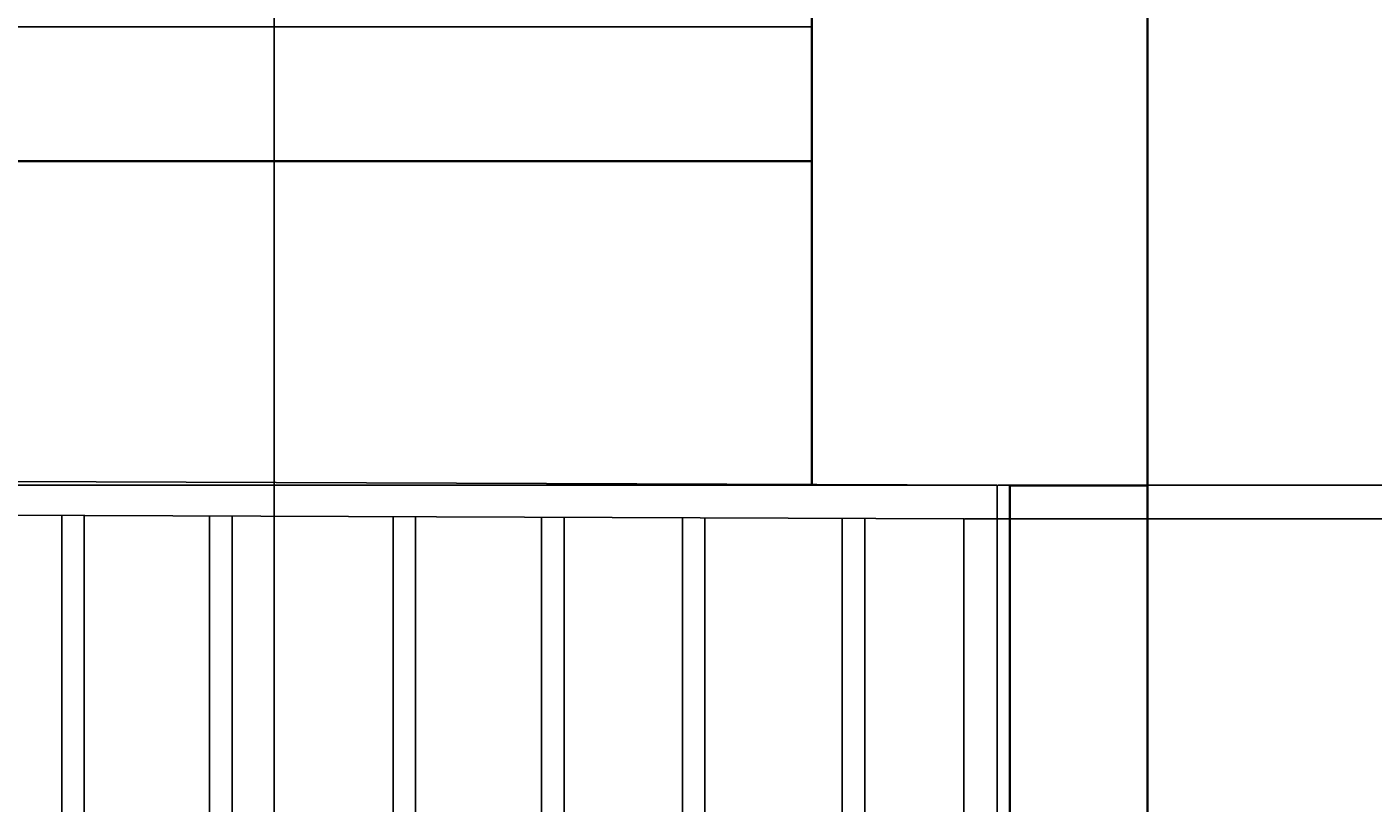
# Model space of a CAD drawing. Units: inches. Extents: x -13 to 809, y 112 to 656.
# Tile 42 of 55: x 521 to 641, y 181 to 251. Entities that reach past the tile are written whole.
import ezdxf

# ---------------------------------------------------------------- set-up
doc = ezdxf.new("R2010")
doc.units = ezdxf.units.IN
doc.header["$MEASUREMENT"] = 0
for name, color, linetype, lineweight in [('A-ANNO-DIMS', 2, 'Continuous', 18), ('A-DOOR', 4, 'Continuous', 25), ('A-ELEV', 7, 'Continuous', 35)]:
    doc.layers.add(name, color=color, linetype=linetype, lineweight=lineweight)
doc.styles.get("Standard").update_dxf_attribs({"font": 'arial.ttf'})
doc.dimstyles.get("Standard").update_dxf_attribs({"dimtxt": 0.625, "dimasz": 0.18, "dimexe": 0.18, "dimexo": 0.0625, "dimgap": 0.09, "dimtad": 0, "dimtih": 1, "dimtoh": 1, "dimdec": 4, "dimzin": 0, "dimdsep": 46, "dimlunit": 4, "dimtxsty": 'Standard', "dimcen": 0.09, "dimadec": 0, "dimazin": 0, "dimtfac": 1, "dimtdec": 4, "dimtofl": 0, "dimtmove": 0, "dimatfit": 3, "dimfxl": 1, "dimtolj": 1, "dimtzin": 0, "dimarcsym": 0})

# ---------------------------------------------------------------- blocks, each defined once
blk = doc.blocks.new('*D20')
at = {"layer": 'A-ANNO-DIMS', "color": 0, "lineweight": -2, "transparency": 16777216}
for p, q in [((365.94, 210.72), (365.94, 112.34)), ((607.57, 209.81), (607.57, 112.34)), ((366.12, 112.52), (485.36, 112.52)), ((607.39, 112.52), (488.15, 112.52))]:
    blk.add_line(p, q, dxfattribs=at)
at = {"layer": 'A-ANNO-DIMS', "color": 0, "transparency": 16777216}
for points in [[(366.12, 112.55), (366.12, 112.49), (365.94, 112.52)], [(607.39, 112.55), (607.39, 112.49), (607.57, 112.52)]]:
    blk.add_solid(points, dxfattribs=at)
at = {"layer": 'Defpoints', "color": 0, "transparency": 16777216}
for p in [(365.94, 210.78), (607.57, 209.88), (607.57, 112.52)]:
    blk.add_point(p, dxfattribs=at)
at = {"layer": 'A-ANNO-DIMS', "color": 0, "transparency": 16777216, "insert": (486.76, 112.52), "char_height": 0.625, "attachment_point": 5}
blk.add_mtext('\\A1;241.64', dxfattribs=at)
blk = doc.blocks.new('*D21')
at = {"layer": 'A-ANNO-DIMS', "color": 0, "lineweight": -2, "transparency": 16777216}
for p, q in [((607.57, 209.81), (607.57, 112.34)), ((621.01, 150.46), (621.01, 112.34)), ((607.75, 112.52), (612.93, 112.52)), ((620.83, 112.52), (615.65, 112.52))]:
    blk.add_line(p, q, dxfattribs=at)
at = {"layer": 'A-ANNO-DIMS', "color": 0, "transparency": 16777216}
for points in [[(607.75, 112.55), (607.75, 112.49), (607.57, 112.52)], [(620.83, 112.55), (620.83, 112.49), (621.01, 112.52)]]:
    blk.add_solid(points, dxfattribs=at)
at = {"layer": 'Defpoints', "color": 0, "transparency": 16777216}
for p in [(607.57, 209.88), (621.01, 150.52), (621.01, 112.52)]:
    blk.add_point(p, dxfattribs=at)
at = {"layer": 'A-ANNO-DIMS', "color": 0, "transparency": 16777216, "insert": (614.29, 112.52), "char_height": 0.625, "attachment_point": 5}
blk.add_mtext('\\A1;13.434', dxfattribs=at)
blk = doc.blocks.new('*D31')
at = {"layer": 'A-ANNO-DIMS', "color": 0, "lineweight": -2, "transparency": 16777216}
for p, q in [((621.07, 617.78), (807.77, 617.78)), ((807.59, 617.6), (807.59, 384.56)), ((807.59, 150.7), (807.59, 383.74)), ((621.07, 150.52), (807.77, 150.52))]:
    blk.add_line(p, q, dxfattribs=at)
at = {"layer": 'A-ANNO-DIMS', "color": 0, "transparency": 16777216}
for points in [[(807.56, 617.6), (807.62, 617.6), (807.59, 617.78)], [(807.56, 150.7), (807.62, 150.7), (807.59, 150.52)]]:
    blk.add_solid(points, dxfattribs=at)
at = {"layer": 'Defpoints', "color": 0, "transparency": 16777216}
for p in [(621.01, 617.78), (807.59, 617.78), (621.01, 150.52)]:
    blk.add_point(p, dxfattribs=at)
at = {"layer": 'A-ANNO-DIMS', "color": 0, "transparency": 16777216, "insert": (807.59, 384.15), "char_height": 0.625, "attachment_point": 5}
blk.add_mtext('\\A1;467.3', dxfattribs=at)
blk = doc.blocks.new('*D49')
at = {"layer": 'A-ANNO-DIMS', "color": 0, "lineweight": -2, "transparency": 16777216}
for p, q in [((590.95, 250.84), (-12.1, 250.84)), ((-11.92, 250.66), (-11.92, 245.25)), ((-11.92, 239.02), (-11.92, 244.44)), ((590.95, 238.84), (-12.1, 238.84))]:
    blk.add_line(p, q, dxfattribs=at)
at = {"layer": 'A-ANNO-DIMS', "color": 0, "transparency": 16777216}
for points in [[(-11.95, 250.66), (-11.89, 250.66), (-11.92, 250.84)], [(-11.95, 239.02), (-11.89, 239.02), (-11.92, 238.84)]]:
    blk.add_solid(points, dxfattribs=at)
at = {"layer": 'Defpoints', "color": 0, "transparency": 16777216}
for p in [(-11.92, 250.84), (591.01, 250.84), (591.01, 238.84)]:
    blk.add_point(p, dxfattribs=at)
at = {"layer": 'A-ANNO-DIMS', "color": 0, "transparency": 16777216, "insert": (-11.92, 244.84), "char_height": 0.625, "attachment_point": 5}
blk.add_mtext('\\A1;12', dxfattribs=at)
blk = doc.blocks.new('*D50')
at = {"layer": 'A-ANNO-DIMS', "color": 0, "lineweight": -2, "transparency": 16777216}
for p, q in [((590.95, 238.84), (-12.1, 238.84)), ((-11.92, 238.66), (-11.92, 224.77)), ((-11.92, 210.06), (-11.92, 223.95)), ((607.51, 209.88), (-12.1, 209.88))]:
    blk.add_line(p, q, dxfattribs=at)
at = {"layer": 'A-ANNO-DIMS', "color": 0, "transparency": 16777216}
for points in [[(-11.95, 238.66), (-11.89, 238.66), (-11.92, 238.84)], [(-11.95, 210.06), (-11.89, 210.06), (-11.92, 209.88)]]:
    blk.add_solid(points, dxfattribs=at)
at = {"layer": 'Defpoints', "color": 0, "transparency": 16777216}
for p in [(591.01, 238.84), (-11.92, 209.88), (607.57, 209.88)]:
    blk.add_point(p, dxfattribs=at)
at = {"layer": 'A-ANNO-DIMS', "color": 0, "transparency": 16777216, "insert": (-11.92, 224.36), "char_height": 0.625, "attachment_point": 5}
blk.add_mtext('\\A1;28.97', dxfattribs=at)
blk = doc.blocks.new('*D52')
at = {"layer": 'A-ANNO-DIMS', "color": 0, "lineweight": -2, "transparency": 16777216}
for p, q in [((442.18, 288.39), (442.18, 112.34)), ((542.96, 288.39), (542.96, 112.34)), ((442.36, 112.52), (491.21, 112.52)), ((542.78, 112.52), (493.93, 112.52))]:
    blk.add_line(p, q, dxfattribs=at)
at = {"layer": 'A-ANNO-DIMS', "color": 0, "transparency": 16777216}
for points in [[(442.36, 112.55), (442.36, 112.49), (442.18, 112.52)], [(542.78, 112.55), (542.78, 112.49), (542.96, 112.52)]]:
    blk.add_solid(points, dxfattribs=at)
at = {"layer": 'Defpoints', "color": 0, "transparency": 16777216}
for p in [(442.18, 288.45), (542.96, 288.45), (542.96, 112.52)]:
    blk.add_point(p, dxfattribs=at)
at = {"layer": 'A-ANNO-DIMS', "color": 0, "transparency": 16777216, "insert": (492.57, 112.52), "char_height": 0.625, "attachment_point": 5}
blk.add_mtext('\\A1;100.78', dxfattribs=at)
blk = doc.blocks.new('*D129')
at = {"layer": 'A-ANNO-DIMS', "color": 0, "lineweight": -2, "transparency": 16777216}
for p, q in [((607.64, 209.88), (807.77, 209.88)), ((807.59, 209.7), (807.59, 180.61)), ((807.59, 150.7), (807.59, 179.79)), ((608.76, 150.52), (807.77, 150.52))]:
    blk.add_line(p, q, dxfattribs=at)
at = {"layer": 'A-ANNO-DIMS', "color": 0, "transparency": 16777216}
for points in [[(807.56, 209.7), (807.62, 209.7), (807.59, 209.88)], [(807.56, 150.7), (807.62, 150.7), (807.59, 150.52)]]:
    blk.add_solid(points, dxfattribs=at)
at = {"layer": 'Defpoints', "color": 0, "transparency": 16777216}
for p in [(607.57, 209.88), (807.59, 209.88), (608.69, 150.52)]:
    blk.add_point(p, dxfattribs=at)
at = {"layer": 'A-ANNO-DIMS', "color": 0, "transparency": 16777216, "insert": (807.59, 180.2), "char_height": 0.625, "attachment_point": 5}
blk.add_mtext('\\A1;59.36', dxfattribs=at)
blk = doc.blocks.new('*D132')
at = {"layer": 'A-ANNO-DIMS', "color": 0, "lineweight": -2, "transparency": 16777216}
for p, q in [((607.64, 209.88), (807.77, 209.88)), ((807.59, 209.7), (807.59, 208.79)), ((807.59, 207.07), (807.59, 207.97)), ((604.64, 206.89), (807.77, 206.89))]:
    blk.add_line(p, q, dxfattribs=at)
at = {"layer": 'A-ANNO-DIMS', "color": 0, "transparency": 16777216}
for points in [[(807.56, 209.7), (807.62, 209.7), (807.59, 209.88)], [(807.56, 207.07), (807.62, 207.07), (807.59, 206.89)]]:
    blk.add_solid(points, dxfattribs=at)
at = {"layer": 'Defpoints', "color": 0, "transparency": 16777216}
for p in [(607.57, 209.88), (807.59, 209.88), (604.57, 206.89)]:
    blk.add_point(p, dxfattribs=at)
at = {"layer": 'A-ANNO-DIMS', "color": 0, "transparency": 16777216, "insert": (807.59, 208.38), "char_height": 0.625, "attachment_point": 5}
blk.add_mtext('\\A1;2.989', dxfattribs=at)

msp = doc.modelspace()

# ---------------------------------------------------------------- linework, layer by layer
at = {"layer": 'A-DOOR'}
for p, q in [((525.9709, 210.19), (525.9709, 210.1825)), ((539.1843, 210.1403), (539.1843, 210.1328)), ((555.5951, 210.0785), (555.5951, 210.071)), ((568.8541, 210.0286), (568.8541, 210.0211)), ((581.4311, 209.9813), (581.4311, 209.9737)), ((523.9709, 207.19), (523.9709, 155.2141)), ((525.9709, 207.1825), (525.9709, 155.2141)), ((537.1843, 207.1403), (537.1843, 155.2141)), ((539.1843, 207.1328), (539.1843, 155.2141)), ((553.5951, 207.0785), (553.5951, 155.2141)), ((555.5951, 207.071), (555.5951, 155.2141)), ((566.8541, 207.0286), (566.8541, 155.2141)), ((568.8541, 207.0211), (568.8541, 155.2141)), ((579.4311, 206.9813), (579.4311, 155.2141)), ((581.4311, 206.9737), (581.4311, 155.2141)), ((593.7248, 206.9274), (593.7248, 155.2141)), ((595.7248, 206.9199), (595.7248, 155.2141))]:
    msp.add_line(p, q, dxfattribs=at)
for points in [[(365.9383, 210.7849), (607.5741, 209.8753), (607.5741, 152.2141), (365.9383, 152.2141)], [(368.9383, 207.7736), (604.5741, 206.8866), (604.5741, 155.2141), (368.9383, 155.2141)]]:
    msp.add_lwpolyline(points, close=True, dxfattribs=at)
at = {"layer": 'A-ELEV'}
for p, q in [((591.008, 209.8635), (591.008, 558.5199)), ((621.008, 209.8635), (621.008, 558.5199)), ((341.4072, 238.8429), (591.008, 238.8429)), ((608.694, 209.8635), (608.694, 150.5199)), ((608.694, 209.8635), (621.008, 209.8635)), ((621.008, 209.8635), (621.008, 150.5199))]:
    msp.add_line(p, q, dxfattribs=at)

# ---------------------------------------------------------------- dimensions: what is measured, and where the dimension line sits
at = {"layer": 'A-ANNO-DIMS'}
for base, p1, p2, override, picture, middle in [((807.5888, 617.7828), (621.008, 150.5199), (621.008, 617.7828), {"dimdec": 1, "dimlfac": 1, "dimrnd": 0, "dimzin": 0, "dimdsep": 46, "dimlunit": 2}, '*D31', (807.5888, 384.1514)), ((-11.9191, 250.8429), (591.008, 238.8429), (591.008, 250.8429), {"dimdec": 0, "dimlfac": 1, "dimrnd": 0, "dimzin": 0, "dimdsep": 46, "dimlunit": 2}, '*D49', (-11.9191, 244.8429)), ((-11.9191, 209.8753), (591.008, 238.8429), (607.5741, 209.8753), {"dimdec": 2, "dimlfac": 1, "dimrnd": 0, "dimzin": 0, "dimdsep": 46, "dimlunit": 2}, '*D50', (-11.9191, 224.3591)), ((807.5888, 209.8753), (604.5741, 206.8866), (607.5741, 209.8753), {"dimdec": 3, "dimlfac": 1, "dimrnd": 0, "dimzin": 0, "dimdsep": 46, "dimlunit": 2}, '*D132', (807.5888, 208.381)), ((807.5888, 209.8753), (608.694, 150.5199), (607.5741, 209.8753), {"dimdec": 2, "dimlfac": 1, "dimrnd": 0, "dimzin": 0, "dimdsep": 46, "dimlunit": 2}, '*D129', (807.5888, 180.1976))]:
    dim = msp.add_linear_dim(base=base, p1=p1, p2=p2, angle=90, dimstyle='Standard', override=override, dxfattribs=at)
    dim.commit()
    dim.dimension.update_dxf_attribs({"geometry": picture, "text_midpoint": middle})
for base, p1, p2, override, picture, middle in [((542.9617, 112.5199), (442.1845, 288.4508), (542.9617, 288.4508), {"dimdec": 2, "dimlfac": 1, "dimrnd": 0, "dimzin": 0, "dimdsep": 46, "dimlunit": 2}, '*D52', (492.5731, 112.5199)), ((607.5741, 112.5199), (365.9383, 210.7849), (607.5741, 209.8753), {"dimdec": 2, "dimlfac": 1, "dimrnd": 0, "dimzin": 0, "dimdsep": 46, "dimlunit": 2}, '*D20', (486.7562, 112.5199)), ((621.008, 112.5199), (607.5741, 209.8753), (621.008, 150.5199), {"dimdec": 3, "dimlfac": 1, "dimrnd": 0, "dimzin": 0, "dimdsep": 46, "dimlunit": 2}, '*D21', (614.2911, 112.5199))]:
    dim = msp.add_linear_dim(base=base, p1=p1, p2=p2, dimstyle='Standard', override=override, dxfattribs=at)
    dim.commit()
    dim.dimension.update_dxf_attribs({"geometry": picture, "text_midpoint": middle})

doc.saveas('drawing.dxf')
